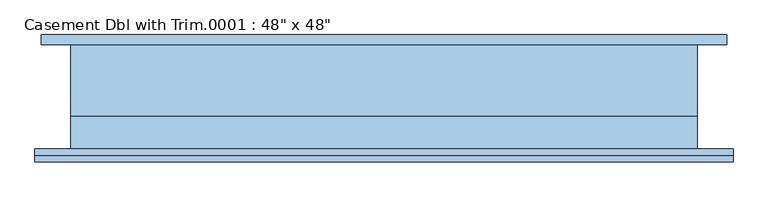
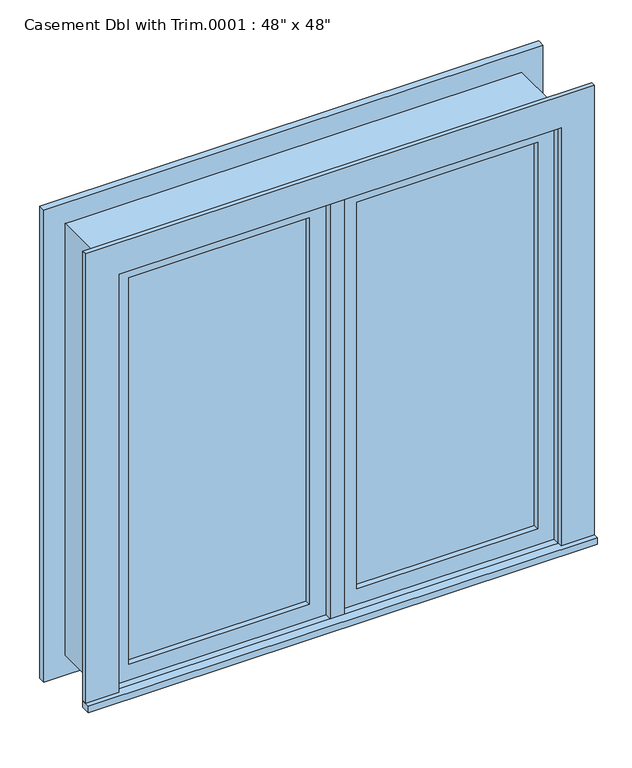
"""IFC4 building model written with IfcOpenShell, lengths in millimetres: window geometry."""

from ifc_helpers import new_model, si_unit, frame, origin, place, context, project, spatial, polyline, outline, extrude, source, transform, mapped, element, save


def window_3a1167bf(model_context):
    return source(origin(), model_context, "Body", "SweptSolid", [
        extrude(outline(polyline([(63.5, -85.725), (63.5, -73.025), (546.1, -73.025), (546.1, -85.725), (63.5, -85.725)])), frame((0.0, 0.0, 977.9), z_axis=(0.0, 0.0, 1.0), x_axis=(1.0, 0.0, 0.0)), (0.0, 0.0, 1.0), 1092.2),
        extrude(outline(polyline([(2114.55, 19.05), (933.45, 19.05), (933.45, 590.55), (2114.55, 590.55), (2114.55, 19.05)]), holes=[polyline([(2070.1, 63.5), (2070.1, 546.1), (977.9, 546.1), (977.9, 63.5), (2070.1, 63.5)])]), frame((0.0, -101.6, 0.0), z_axis=(0.0, 1.0, 0.0), x_axis=(0.0, 0.0, 1.0)), (0.0, 0.0, 1.0), 44.45),
        extrude(outline(polyline([(19.05, -57.15), (19.05, -120.65), (-19.05, -120.65), (-19.05, -57.15), (19.05, -57.15)])), frame((0.0, 0.0, 933.45), z_axis=(0.0, 0.0, 1.0), x_axis=(1.0, 0.0, 0.0)), (0.0, 0.0, 1.0), 1181.1),
        extrude(outline(polyline([(-679.45, -146.05), (-679.45, -120.65), (679.45, -120.65), (679.45, -146.05), (-679.45, -146.05)])), frame((0.0, 0.0, 914.4), z_axis=(0.0, 0.0, 1.0), x_axis=(1.0, 0.0, 0.0)), (0.0, 0.0, 1.0), 19.05),
        extrude(outline(polyline([(2114.55, -590.55), (2114.55, 590.55), (933.45, 590.55), (933.45, 679.45), (2203.45, 679.45), (2203.45, -679.45), (933.45, -679.45), (933.45, -590.55), (2114.55, -590.55)])), frame((0.0, -133.35, 0.0), z_axis=(0.0, 1.0, 0.0), x_axis=(0.0, 0.0, 1.0)), (0.0, 0.0, 1.0), 12.7),
        extrude(outline(polyline([(2190.75, 666.75), (2190.75, -666.75), (857.25, -666.75), (857.25, 666.75), (2190.75, 666.75)]), holes=[polyline([(2101.85, 577.85), (946.15, 577.85), (946.15, -577.85), (2101.85, -577.85), (2101.85, 577.85)])]), frame((0.0, 82.55, 0.0), z_axis=(0.0, 1.0, 0.0), x_axis=(0.0, 0.0, 1.0)), (0.0, 0.0, 1.0), 19.05),
        extrude(outline(polyline([(-63.5, -73.025), (-63.5, -85.725), (-546.1, -85.725), (-546.1, -73.025), (-63.5, -73.025)])), frame((0.0, 0.0, 977.9), z_axis=(0.0, 0.0, 1.0), x_axis=(1.0, 0.0, 0.0)), (0.0, 0.0, 1.0), 1092.2),
        extrude(outline(polyline([(2114.55, -590.55), (933.45, -590.55), (933.45, -19.05), (2114.55, -19.05), (2114.55, -590.55)]), holes=[polyline([(2070.1, -546.1), (2070.1, -63.5), (977.9, -63.5), (977.9, -546.1), (2070.1, -546.1)])]), frame((0.0, -101.6, 0.0), z_axis=(0.0, 1.0, 0.0), x_axis=(0.0, 0.0, 1.0)), (0.0, 0.0, 1.0), 44.45),
        extrude(outline(polyline([(2133.6, -609.6), (914.4, -609.6), (914.4, 609.6), (2133.6, 609.6), (2133.6, -609.6)]), holes=[polyline([(2101.85, -577.85), (2101.85, 577.85), (946.15, 577.85), (946.15, -577.85), (2101.85, -577.85)])]), frame((0.0, -57.15, 0.0), z_axis=(0.0, 1.0, 0.0), x_axis=(0.0, 0.0, 1.0)), (0.0, 0.0, 1.0), 139.7),
        extrude(outline(polyline([(2133.6, 609.6), (2133.6, -609.6), (914.4, -609.6), (914.4, 609.6), (2133.6, 609.6)]), holes=[polyline([(2114.55, 590.55), (933.45, 590.55), (933.45, -590.55), (2114.55, -590.55), (2114.55, 590.55)])]), frame((0.0, -120.65, 0.0), z_axis=(0.0, 1.0, 0.0), x_axis=(0.0, 0.0, 1.0)), (0.0, 0.0, 1.0), 63.5),
    ])


if __name__ == "__main__":
    model = new_model("IFC4")
    model_context = context("Model", 3, world=origin())
    ifc_project = project(units=[si_unit("LENGTHUNIT", "METRE", prefix="MILLI")], contexts=[model_context])
    site = spatial("IfcSite", under=ifc_project)
    building = spatial("IfcBuilding", under=site)
    placement = place(None, origin())
    window_shape = window_3a1167bf(model_context)
    element("IfcWindow", 1, ObjectType="Casement Dbl with Trim.0001 : 48\" x 48\"", at=placement, inside=building, context=model_context, shape_type="MappedRepresentation", body=[
        mapped(window_shape, transform((0.0, 0.0, 0.0), x_axis=(1.0, 0.0, 0.0), y_axis=(0.0, 1.0, 0.0), z_axis=(0.0, 0.0, 1.0))),
    ])
    save(model, "model.ifc")

# Revit data of these elements
# Type "Casement Dbl with Trim.0001 : 48\" x 48\""
#   Type Mark = "23"
#   Construction Type Id = "GSP4R"
#   Assembly Code = "B2020100"
#   Analytic Construction = "1/8 in Pilkington single glazing"
#   Visual Light Transmittance = 0.9
#   Solar Heat Gain Coefficient = 0.78
#   Heat Transfer Coefficient (U) = 0.6496 BTU/(h·ft²·°F)
#   Height = 4' - 0"
#   Default Sill Height = 3' - 0"
#   Trim Projection - Ext. = 0' - 0 1/2"
#   Trim Projection - Int. = 0' - 0 3/4"
#   Trim Width - Exterior = 0' - 3 1/2"
#   Trim Width - Interior = 0' - 3 1/2"
#   Width = 4' - 0"
#   Window Inset = 0' - 0 3/4"
#   Define Thermal Properties by = 1
#   Glass Pane Material = Glass
#   Sash Material = Sash
#   Trim Exterior Material = Trim
#   Trim Interior Material = Trim
#   Wall Closure = (empty or 0)
# Element 1 (IfcWindow, "Casement Dbl with Trim.0001 : 48\" x 48\"")
#   Materials on its faces: "Sash", "Trim", "Glass"
# Materials
#   "Glass": class "Glass", colour RGB 0 128 192, transparency 0.75, Description = "Soda Lime Glass", Cost = 0
#   "Sash": class "Wood", colour RGB 224 178 126, transparency 0
#   "Trim": class "Wood", colour RGB 224 178 126, transparency 0
